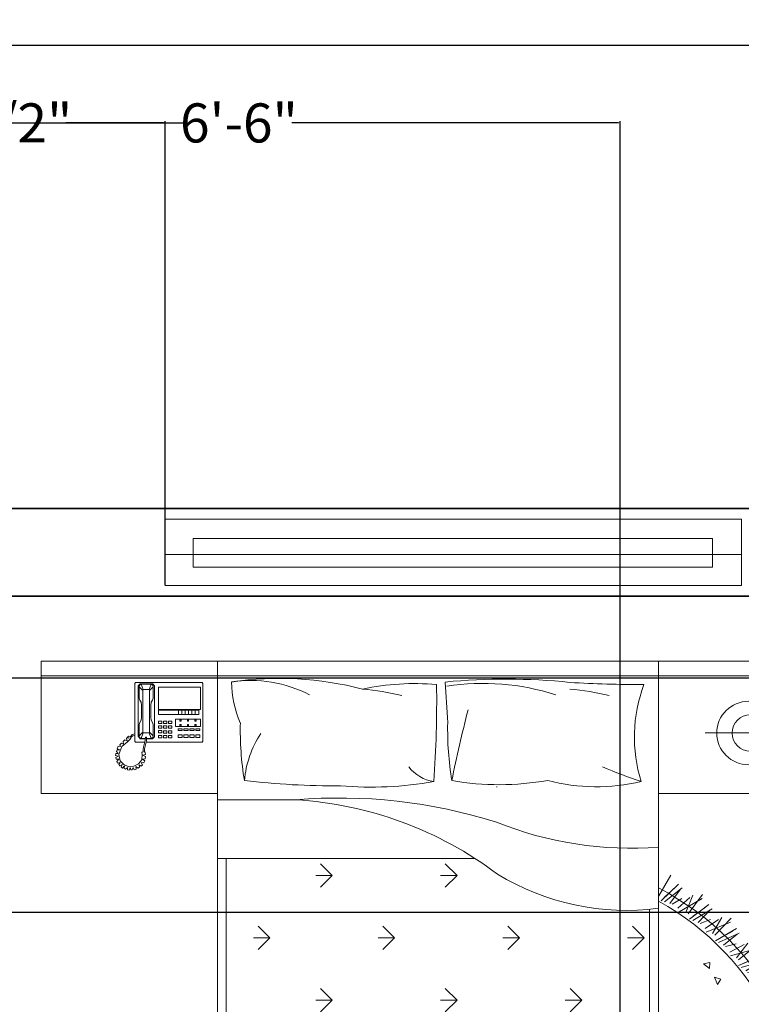
# Model space of a CAD drawing. Units: inches. Extents: x 311 to 754, y 60 to 497.
# Tile 4 of 11: x 388 to 462, y 396 to 497. Entities that reach past the tile are written whole.
import ezdxf

# ---------------------------------------------------------------- set-up
doc = ezdxf.new("R2010")
doc.units = ezdxf.units.IN
doc.header["$MEASUREMENT"] = 0
for name, color, linetype, lineweight in [('A-ANNO-DIMS', 2, 'Continuous', 18), ('A-WALL', 7, 'Continuous', 35), ('beds', 70, 'Continuous', 13), ('windows', 120, 'Continuous', 18)]:
    doc.layers.add(name, color=color, linetype=linetype, lineweight=lineweight)
doc.styles.get("Standard").update_dxf_attribs({"font": 'arial.ttf'})
doc.dimstyles.get("Standard").update_dxf_attribs({"dimtxt": 4, "dimasz": 0.18, "dimexe": 0.18, "dimexo": 0.0625, "dimgap": 0.09, "dimtad": 0, "dimtih": 1, "dimtoh": 1, "dimdec": 0, "dimrnd": 6, "dimzin": 0, "dimdsep": 46, "dimlunit": 3, "dimtxsty": 'Standard', "dimcen": 0.09, "dimadec": 0, "dimazin": 0, "dimtfac": 1, "dimtdec": 0, "dimtofl": 0, "dimtmove": 0, "dimatfit": 3, "dimfxl": 1, "dimtolj": 1, "dimtzin": 0, "dimarcsym": 0})

# ---------------------------------------------------------------- blocks, each defined once
blk = doc.blocks.new('A$C57792D97')
for p, q in [((0.6, 2.6235), (0, 2.6235)), ((0, 2.6235), (0, 2.1735)), ((2.1, 2.6235), (0.6, 2.6235)), ((0.6, 2.6235), (0.6, 0.6235)), ((0.6, 0.6235), (0.6, 2.6235)), ((0.6, 2.1735), (0.6, 2.6235)), ((2.1, 0.6235), (2.1, 2.6235)), ((2.7, 2.6235), (2.1, 2.6235)), ((2.1, 2.6235), (2.1, 2.1735)), ((2.7, 2.1735), (2.7, 2.6235)), ((0.6, 2.5735), (0, 2.5735)), ((2.1, 2.5735), (0.6, 2.5735)), ((2.7, 2.5735), (2.1, 2.5735)), ((2.4103, 2.2312), (2.4103, 2.5317)), ((2.2593, 2.3802), (2.5698, 2.3802)), ((1.5491, 2.1955), (1.5516, 2.1955)), ((0, 2.1735), (0.6, 2.1735)), ((0.6, 2.1518), (0.8661, 2.1518)), ((2.1, 2.1735), (2.7, 2.1735)), ((0.6, 1.9518), (1.4767, 1.9518)), ((0.63, 0.6535), (0.63, 1.9518)), ((0.9906, 1.8942), (0.9508, 1.934)), ((1.4149, 1.8942), (1.3751, 1.934)), ((0.9906, 1.8942), (0.9344, 1.8942)), ((0.9906, 1.8942), (0.9508, 1.8544)), ((1.4149, 1.8942), (1.3586, 1.8942)), ((1.4149, 1.8942), (1.3751, 1.8544)), ((2.142, 1.8959), (2.1018, 1.8254)), ((2.1679, 1.8652), (2.1088, 1.8077)), ((2.1584, 1.8544), (2.1201, 1.8188)), ((2.1812, 1.8524), (2.1207, 1.8046)), ((2.1749, 1.8475), (2.1394, 1.7993)), ((2.1799, 1.8155), (2.1465, 1.7971)), ((2.2066, 1.8191), (2.1664, 1.7827)), ((2.249, 1.8154), (2.1711, 1.7709)), ((2.2173, 1.8274), (2.1931, 1.7688)), ((2.2496, 1.8292), (2.2008, 1.7642)), ((2.07, 1.7793), (2.07, 0.6535)), ((2.2713, 1.7954), (2.2055, 1.7458)), ((2.283, 1.7811), (2.2169, 1.7413)), ((2.2607, 1.7859), (2.2181, 1.7554)), ((2.2761, 1.777), (2.2348, 1.7337)), ((2.277, 1.7446), (2.2416, 1.7306)), ((2.304, 1.7449), (2.2596, 1.7138)), ((2.3157, 1.7518), (2.2843, 1.6966)), ((2.3479, 1.7495), (2.2914, 1.6911)), ((0.7785, 1.6821), (0.7387, 1.7219)), ((1.2027, 1.6821), (1.163, 1.7219)), ((1.627, 1.6821), (1.5872, 1.7219)), ((2.0513, 1.6821), (2.0115, 1.7219)), ((2.3456, 1.7359), (2.2627, 1.7015)), ((2.3653, 1.7133), (2.2937, 1.6723)), ((0.7785, 1.6821), (0.7222, 1.6821)), ((0.7785, 1.6821), (0.7387, 1.6423)), ((1.2027, 1.6821), (1.1465, 1.6821)), ((1.2027, 1.6821), (1.163, 1.6423)), ((1.627, 1.6821), (1.5708, 1.6821)), ((1.627, 1.6821), (1.5872, 1.6423)), ((2.0513, 1.6821), (1.995, 1.6821)), ((2.0513, 1.6821), (2.0115, 1.6423)), ((2.3751, 1.6976), (2.3045, 1.6664)), ((2.3535, 1.7051), (2.3075, 1.6802)), ((2.3677, 1.6944), (2.3213, 1.6565)), ((2.3645, 1.6621), (2.3277, 1.6526)), ((2.3913, 1.659), (2.3434, 1.6337)), ((2.4314, 1.6449), (2.3449, 1.6211)), ((2.4038, 1.6644), (2.3657, 1.6136)), ((2.4355, 1.6581), (2.372, 1.6073)), ((2.4482, 1.62), (2.372, 1.5882)), ((2.4354, 1.6134), (2.3867, 1.5944)), ((2.2754, 1.598), (2.2534, 1.5939)), ((2.2736, 1.5771), (2.2535, 1.594)), ((2.2736, 1.5771), (2.2754, 1.598)), ((2.4559, 1.6032), (2.382, 1.581)), ((2.4482, 1.6009), (2.3974, 1.5692)), ((2.3123, 1.541), (2.2911, 1.5481)), ((2.3006, 1.5236), (2.2912, 1.5481)), ((2.441, 1.5693), (2.4032, 1.5645)), ((2.4672, 1.5629), (2.4164, 1.5438)), ((2.5052, 1.5438), (2.4164, 1.5311)), ((2.4802, 1.5667), (2.4361, 1.5211)), ((2.5109, 1.5564), (2.4416, 1.514)), ((0.9906, 1.47), (0.9508, 1.5097)), ((1.4149, 1.47), (1.3751, 1.5097)), ((1.8391, 1.47), (1.7994, 1.5097)), ((2.3006, 1.5236), (2.3123, 1.541)), ((2.5187, 1.517), (2.4392, 1.4951)), ((2.5052, 1.5121), (2.4545, 1.4994)), ((2.5243, 1.4994), (2.4482, 1.4867)), ((2.5163, 1.4981), (2.462, 1.473)), ((0.9906, 1.47), (0.9344, 1.47)), ((0.9906, 1.47), (0.9508, 1.4302)), ((1.4149, 1.47), (1.3586, 1.47)), ((1.4149, 1.47), (1.3751, 1.4302)), ((1.8391, 1.47), (1.7829, 1.47)), ((1.8391, 1.47), (1.7994, 1.4302)), ((2.5052, 1.4677), (2.4672, 1.4677)), ((2.5304, 1.458), (2.4777, 1.4454)), ((2.5438, 1.4601), (2.4943, 1.4204)), ((2.573, 1.4461), (2.4989, 1.4127)), ((2.5658, 1.4343), (2.4761, 1.4328)), ((2.5758, 1.406), (2.4942, 1.3942)), ((2.5791, 1.3878), (2.502, 1.3848)), ((2.5618, 1.4028), (2.5099, 1.3966)), ((2.571, 1.3876), (2.514, 1.3695)), ((2.2534, 1.3469), (2.2315, 1.3429)), ((2.2516, 1.326), (2.2315, 1.3429)), ((2.2516, 1.326), (2.2535, 1.347)), ((2.5562, 1.3587), (2.5185, 1.3635)), ((2.58, 1.346), (2.5261, 1.3402)), ((2.5936, 1.3464), (2.5395, 1.3132)), ((2.1596, 1.3147), (2.1502, 1.3392)), ((2.1714, 1.3321), (2.1502, 1.3392)), ((2.1596, 1.3147), (2.1714, 1.3321)), ((2.3632, 1.3229), (2.33, 1.319)), ((2.3584, 1.2918), (2.33, 1.319)), ((2.3584, 1.2918), (2.3632, 1.3229)), ((2.6121, 1.3181), (2.523, 1.3279)), ((2.6207, 1.3289), (2.5431, 1.305)), ((0.7785, 1.2578), (0.7387, 1.2976)), ((1.2027, 1.2578), (1.163, 1.2976)), ((1.627, 1.2578), (1.5872, 1.2976)), ((2.0513, 1.2578), (2.0115, 1.2976)), ((2.6185, 1.2888), (2.5361, 1.2873)), ((2.6195, 1.2703), (2.5426, 1.277)), ((2.6042, 1.2873), (2.5519, 1.2877)), ((0.7785, 1.2578), (0.7222, 1.2578)), ((0.7785, 1.2578), (0.7387, 1.218)), ((1.2027, 1.2578), (1.1465, 1.2578)), ((1.2027, 1.2578), (1.163, 1.218)), ((1.627, 1.2578), (1.5708, 1.2578)), ((1.627, 1.2578), (1.5872, 1.218)), ((2.0513, 1.2578), (1.995, 1.2578)), ((2.0513, 1.2578), (2.0115, 1.218)), ((2.4134, 1.2295), (2.404, 1.254)), ((2.4252, 1.2469), (2.404, 1.254)), ((2.4134, 1.2295), (2.4252, 1.2469)), ((2.6115, 1.2711), (2.5526, 1.2603)), ((2.5932, 1.2443), (2.5563, 1.2538)), ((2.6435, 1.197), (2.5563, 1.2178)), ((2.6152, 1.2287), (2.561, 1.2296)), ((2.6287, 1.2274), (2.5709, 1.2013)), ((2.6462, 1.1671), (2.5642, 1.176)), ((2.6534, 1.2066), (2.5734, 1.1926)), ((2.6319, 1.1675), (2.58, 1.1743)), ((2.4947, 1.1445), (2.4728, 1.1404)), ((2.4929, 1.1236), (2.4728, 1.1404)), ((2.4929, 1.1236), (2.4948, 1.1445)), ((2.6449, 1.1486), (2.5694, 1.1649)), ((2.637, 1.1504), (2.5773, 1.147)), ((2.6155, 1.1261), (2.5801, 1.1402)), ((2.6353, 1.1079), (2.5817, 1.1156)), ((0.9906, 1.0457), (0.9508, 1.0855)), ((1.4149, 1.0457), (1.3751, 1.0855)), ((1.8391, 1.0457), (1.7994, 1.0855)), ((2.2315, 1.0959), (2.2095, 1.0919)), ((2.2297, 1.075), (2.2096, 1.0919)), ((2.2297, 1.075), (2.2315, 1.0959)), ((2.6595, 1.0729), (2.5756, 1.1045)), ((2.6486, 1.1049), (2.588, 1.0862)), ((2.6705, 1.0812), (2.5894, 1.0774)), ((0.9906, 1.0457), (0.9344, 1.0457)), ((0.9906, 1.0457), (0.9508, 1.0059)), ((1.4149, 1.0457), (1.3586, 1.0457)), ((1.4149, 1.0457), (1.3751, 1.0059)), ((1.8391, 1.0457), (1.7829, 1.0457)), ((1.8391, 1.0457), (1.7994, 1.0059)), ((2.2725, 1.0206), (2.2631, 1.0451)), ((2.2842, 1.038), (2.2631, 1.0451)), ((2.6584, 1.0429), (2.5782, 1.062)), ((2.6548, 1.0248), (2.582, 1.0503)), ((2.6442, 1.045), (2.5937, 1.0584)), ((2.2725, 1.0206), (2.2843, 1.038)), ((2.6472, 1.0275), (2.5875, 1.0316)), ((2.6228, 1.0061), (2.5895, 1.0244)), ((2.6598, 0.9477), (2.5805, 0.9897)), ((2.6402, 0.9855), (2.588, 0.9999)), ((2.653, 0.9809), (2.5905, 0.97)), ((2.3053, 0.9493), (2.272, 0.9455)), ((2.3005, 0.9182), (2.2721, 0.9455)), ((2.3005, 0.9182), (2.3053, 0.9494)), ((2.5263, 0.9355), (2.5169, 0.96)), ((2.538, 0.9528), (2.5169, 0.9599)), ((2.5263, 0.9355), (2.5381, 0.9529)), ((2.655, 0.9181), (2.5778, 0.9471)), ((2.6718, 0.9546), (2.5908, 0.961)), ((2.6412, 0.9221), (2.5927, 0.9416)), ((2.6491, 0.9006), (2.5801, 0.9351)), ((2.6419, 0.9043), (2.5832, 0.9159)), ((2.6151, 0.8861), (2.5843, 0.9085)), ((0.7785, 0.8336), (0.7387, 0.8733)), ((1.2027, 0.8336), (1.163, 0.8733)), ((1.627, 0.8336), (1.5872, 0.8733)), ((2.0513, 0.8336), (2.0115, 0.8733)), ((2.4728, 0.8934), (2.4508, 0.8894)), ((2.471, 0.8725), (2.4509, 0.8894)), ((2.471, 0.8725), (2.4728, 0.8934)), ((2.6444, 0.8236), (2.571, 0.8751)), ((2.6297, 0.8635), (2.5797, 0.8843)), ((2.2095, 0.8449), (2.1876, 0.8408)), ((2.2077, 0.824), (2.1876, 0.8408)), ((2.2077, 0.824), (2.2095, 0.8449)), ((2.6572, 0.8289), (2.5776, 0.8454)), ((2.6418, 0.8573), (2.5785, 0.8543)), ((0.7785, 0.8336), (0.7222, 0.8336)), ((0.7785, 0.8336), (0.7387, 0.7938)), ((1.2027, 0.8336), (1.1465, 0.8336)), ((1.2027, 0.8336), (1.163, 0.7938)), ((1.627, 0.8336), (1.5708, 0.8336)), ((1.627, 0.8336), (1.5872, 0.7938)), ((2.0513, 0.8336), (1.995, 0.8336)), ((2.0513, 0.8336), (2.0115, 0.7938)), ((2.1316, 0.8117), (2.1222, 0.8362)), ((2.1433, 0.8291), (2.1222, 0.8362)), ((2.1316, 0.8117), (2.1434, 0.8291)), ((2.6359, 0.7948), (2.5629, 0.8332)), ((2.6279, 0.7781), (2.5637, 0.821)), ((2.6227, 0.8004), (2.577, 0.8259)), ((1.9462, 0.7963), (1.9243, 0.7923)), ((2.6212, 0.7827), (2.5644, 0.8015)), ((2.5923, 0.768), (2.5646, 0.7941)), ((1.683, 0.7477), (1.661, 0.7437)), ((2.3854, 0.7265), (2.376, 0.751)), ((2.3971, 0.7439), (2.376, 0.751)), ((2.3854, 0.7265), (2.3972, 0.7439)), ((2.6136, 0.7023), (2.5472, 0.7626)), ((2.6153, 0.7361), (2.552, 0.7411)), ((2.604, 0.7437), (2.557, 0.7707)), ((2.5915, 0.6593), (2.5332, 0.7099)), ((2.6016, 0.6748), (2.534, 0.7221)), ((2.5892, 0.6821), (2.547, 0.7131)), ((2.6269, 0.706), (2.5501, 0.7323)), ((1.4197, 0.6992), (1.3978, 0.6951)), ((2.5549, 0.6537), (2.5307, 0.6831)), ((2.5855, 0.6646), (2.5315, 0.6905)), ((0.9906, 0.6214), (0.9508, 0.6612)), ((1.1564, 0.6506), (1.1345, 0.6466)), ((1.4149, 0.6214), (1.3751, 0.6612)), ((1.8391, 0.6214), (1.7994, 0.6612)), ((2.4508, 0.6424), (2.4289, 0.6383)), ((2.449, 0.6215), (2.4289, 0.6384)), ((2.449, 0.6215), (2.4508, 0.6424)), ((2.5678, 0.5858), (2.5095, 0.654)), ((2.5635, 0.6282), (2.5203, 0.6608)), ((2.02, 0.6035), (0.6716, 0.6035)), ((0.9906, 0.6214), (0.9344, 0.6214)), ((0.9906, 0.6214), (0.9727, 0.6035)), ((1.4149, 0.6214), (1.3586, 0.6214)), ((1.4149, 0.6214), (1.397, 0.6035)), ((1.8391, 0.6214), (1.7829, 0.6214)), ((1.8391, 0.6214), (1.8212, 0.6035)), ((2.5405, 0.546), (2.489, 0.6034)), ((2.5524, 0.5601), (2.4913, 0.6155)), ((2.541, 0.5688), (2.5031, 0.6049)), ((2.5815, 0.5878), (2.5085, 0.6236)), ((2.5737, 0.6192), (2.5116, 0.632)), ((0.6417, 0.5735), (2.05, 0.5735)), ((0.8932, 0.6021), (0.8712, 0.598)), ((1.3422, 0.5642), (1.3386, 0.5735)), ((1.3422, 0.5642), (1.3485, 0.5735)), ((2.1875, 0.5938), (2.1656, 0.5898)), ((2.1857, 0.5729), (2.1656, 0.5898)), ((2.1857, 0.5729), (2.1876, 0.5938)), ((2.2473, 0.5758), (2.2141, 0.5719)), ((2.2425, 0.5447), (2.2141, 0.572)), ((2.2425, 0.5447), (2.2474, 0.5758)), ((2.5035, 0.545), (2.4831, 0.5772)), ((2.5352, 0.552), (2.4849, 0.5844)), ((0.8142, 0.5177), (0.8685, 0.5428)), ((1.9243, 0.5453), (1.9023, 0.5412)), ((1.9225, 0.5244), (1.9024, 0.5412)), ((1.9225, 0.5244), (1.9243, 0.5453)), ((2.2445, 0.5176), (2.2351, 0.5421)), ((2.5078, 0.476), (2.4585, 0.551)), ((2.5088, 0.5186), (2.47, 0.5564)), ((0.8062, 0.5164), (0.8823, 0.5291)), ((0.8118, 0.4988), (0.8913, 0.5207)), ((0.8253, 0.5037), (0.876, 0.5164)), ((1.6077, 0.4964), (1.5865, 0.5035)), ((1.596, 0.479), (1.5866, 0.5035)), ((1.8485, 0.5294), (1.8152, 0.5255)), ((1.8437, 0.4983), (1.8153, 0.5256)), ((1.8437, 0.4983), (1.8485, 0.5294)), ((2.2445, 0.5176), (2.2562, 0.535)), ((2.4757, 0.4399), (2.4318, 0.5034)), ((2.4893, 0.4525), (2.4356, 0.515)), ((2.4791, 0.4625), (2.446, 0.503)), ((2.5216, 0.4763), (2.4537, 0.5209)), ((2.5178, 0.5084), (2.4578, 0.5289)), ((0.8196, 0.4594), (0.8889, 0.5018)), ((0.8253, 0.472), (0.9141, 0.4847)), ((0.8503, 0.4491), (0.8944, 0.4947)), ((0.8633, 0.4529), (0.9141, 0.472)), ((1.4496, 0.483), (1.4163, 0.4791)), ((1.4448, 0.4519), (1.4164, 0.4792)), ((1.4448, 0.4519), (1.4496, 0.483)), ((1.596, 0.479), (1.6077, 0.4964)), ((1.661, 0.4967), (1.6391, 0.4927)), ((1.6592, 0.4758), (1.6391, 0.4927)), ((1.6592, 0.4758), (1.661, 0.4967)), ((2.4389, 0.4436), (2.4227, 0.478)), ((2.4712, 0.4466), (2.4253, 0.485)), ((0.8823, 0.4149), (0.9331, 0.4466)), ((0.8895, 0.4465), (0.9273, 0.4513)), ((0.9592, 0.4578), (0.938, 0.4649)), ((0.9403, 0.459), (0.9381, 0.4649)), ((0.9508, 0.4454), (0.9592, 0.4578)), ((1.0507, 0.4366), (1.0175, 0.4327)), ((1.0459, 0.4055), (1.0507, 0.4366)), ((1.3977, 0.4481), (1.3758, 0.4441)), ((1.3959, 0.4272), (1.3758, 0.4441)), ((1.3959, 0.4272), (1.3978, 0.4482)), ((2.4345, 0.3746), (2.395, 0.4552)), ((2.4409, 0.4167), (2.4071, 0.4591)), ((0.8746, 0.4126), (0.9485, 0.4347)), ((0.8823, 0.3958), (0.9585, 0.4275)), ((0.895, 0.3577), (0.9585, 0.4085)), ((0.8951, 0.4024), (0.9438, 0.4214)), ((1.0459, 0.4055), (1.0175, 0.4328)), ((1.8615, 0.4113), (1.8403, 0.4184)), ((1.8498, 0.3939), (1.8404, 0.4184)), ((1.8498, 0.3939), (1.8615, 0.4113)), ((2.3981, 0.3428), (2.3625, 0.4113)), ((2.4132, 0.3535), (2.3678, 0.4224)), ((2.4043, 0.3648), (2.3766, 0.4092)), ((2.4482, 0.3731), (2.3865, 0.4259)), ((2.4485, 0.4055), (2.3915, 0.4334)), ((0.8991, 0.3709), (0.9856, 0.3946)), ((0.9267, 0.3514), (0.9648, 0.4022)), ((0.9392, 0.3568), (0.9872, 0.3821)), ((1.1345, 0.3996), (1.1125, 0.3955)), ((1.1327, 0.3787), (1.1126, 0.3955)), ((1.1327, 0.3787), (1.1345, 0.3996)), ((1.213, 0.3727), (1.1918, 0.3798)), ((1.2013, 0.3553), (1.1919, 0.3798)), ((1.2013, 0.3553), (1.213, 0.3727)), ((2.3607, 0.3242), (2.3324, 0.3704)), ((2.3621, 0.3511), (2.3503, 0.3873)), ((2.3945, 0.35), (2.3538, 0.3939)), ((0.9555, 0.3182), (1.026, 0.3494)), ((0.9628, 0.3214), (1.0092, 0.3592)), ((0.9652, 0.3025), (1.0368, 0.3435)), ((0.966, 0.3537), (1.0029, 0.3631)), ((0.977, 0.3107), (1.023, 0.3356)), ((2.1656, 0.3428), (2.1436, 0.3387)), ((2.1638, 0.3219), (2.1437, 0.3388)), ((2.1638, 0.3219), (2.1656, 0.3428)), ((2.3253, 0.265), (2.2888, 0.3389)), ((2.3625, 0.28), (2.3078, 0.3401)), ((2.3668, 0.3121), (2.3138, 0.3469)), ((2.3491, 0.2832), (2.32, 0.3681)), ((0.9826, 0.2663), (1.0392, 0.3246)), ((0.9849, 0.2799), (1.0678, 0.3143)), ((1.0148, 0.264), (1.0462, 0.3191)), ((1.0265, 0.2709), (1.0709, 0.302)), ((2.1153, 0.3261), (2.0941, 0.3332)), ((2.1036, 0.3087), (2.0942, 0.3332)), ((2.1036, 0.3087), (2.1153, 0.3261)), ((2.2743, 0.2689), (2.2671, 0.3063)), ((2.3063, 0.2638), (2.2714, 0.3124)), ((2.309, 0.2562), (2.2823, 0.3286)), ((2.3179, 0.2773), (2.2959, 0.3247)), ((1.0475, 0.2347), (1.1136, 0.2745)), ((1.0535, 0.2712), (1.0889, 0.2852)), ((1.0544, 0.2388), (1.0957, 0.2821)), ((1.0592, 0.2203), (1.125, 0.27)), ((1.4668, 0.2875), (1.4456, 0.2946)), ((1.4551, 0.2701), (1.4457, 0.2946)), ((1.4551, 0.2701), (1.4668, 0.2875)), ((1.9023, 0.2942), (1.8804, 0.2902)), ((1.9005, 0.2733), (1.8804, 0.2902)), ((1.9005, 0.2733), (1.9023, 0.2942)), ((2.2741, 0.2296), (2.2258, 0.2708)), ((2.2529, 0.2032), (2.2346, 0.291)), ((2.2695, 0.2424), (2.2473, 0.2918)), ((1.0699, 0.2299), (1.1124, 0.2604)), ((1.0809, 0.1866), (1.1297, 0.2516)), ((1.0815, 0.2004), (1.1594, 0.2449)), ((1.1132, 0.1884), (1.1374, 0.247)), ((1.639, 0.2457), (1.6171, 0.2416)), ((1.6372, 0.2248), (1.6171, 0.2416)), ((1.6372, 0.2248), (1.6391, 0.2457)), ((2.1768, 0.1984), (2.1745, 0.2364)), ((2.208, 0.1893), (2.1795, 0.2419)), ((2.2097, 0.1814), (2.1923, 0.2566)), ((2.227, 0.1881), (2.2001, 0.2661)), ((2.2212, 0.2012), (2.2053, 0.2511)), ((2.2658, 0.1984), (2.2191, 0.2649)), ((1.1239, 0.1967), (1.1641, 0.2331)), ((1.1493, 0.1634), (1.2098, 0.2112)), ((1.1507, 0.2003), (1.184, 0.2187)), ((1.1556, 0.1683), (1.1911, 0.2165)), ((1.1626, 0.1506), (1.2217, 0.2081)), ((1.7206, 0.2023), (1.6994, 0.2094)), ((1.7089, 0.1849), (1.6995, 0.2095)), ((1.7089, 0.1849), (1.7206, 0.2024)), ((2.1198, 0.1242), (2.1029, 0.2049)), ((2.1596, 0.1295), (2.1216, 0.2013)), ((2.1718, 0.1594), (2.129, 0.2063)), ((2.1474, 0.1359), (2.1403, 0.2253)), ((2.1688, 0.1727), (2.1529, 0.2245)), ((1.1721, 0.1614), (1.2104, 0.197)), ((1.1873, 0.1336), (1.259, 0.1875)), ((1.1885, 0.1199), (1.2287, 0.1904)), ((1.2203, 0.1256), (1.237, 0.1868)), ((1.2299, 0.1352), (1.2652, 0.1764)), ((1.3758, 0.1971), (1.3538, 0.193)), ((1.374, 0.1762), (1.3539, 0.1931)), ((1.374, 0.1762), (1.3758, 0.1971)), ((2.0343, 0.0824), (2.0385, 0.172)), ((2.0601, 0.1162), (2.0509, 0.1696)), ((2.0714, 0.1407), (2.0737, 0.1787)), ((2.1011, 0.1277), (2.0794, 0.1835)), ((2.1018, 0.1197), (2.0939, 0.1965)), ((2.1157, 0.1379), (2.1062, 0.1893)), ((1.2559, 0.1422), (1.2867, 0.1646)), ((1.2592, 0.1054), (1.3133, 0.1604)), ((1.2649, 0.111), (1.2941, 0.1633)), ((1.2741, 0.0944), (1.3255, 0.1588)), ((1.282, 0.1063), (1.3156, 0.1464)), ((1.3007, 0.0806), (1.3651, 0.1431)), ((1.3035, 0.0671), (1.3346, 0.1421)), ((1.3344, 0.0768), (1.3433, 0.1396)), ((1.7905, 0.1559), (1.7573, 0.152)), ((1.7857, 0.1248), (1.7573, 0.152)), ((1.7857, 0.1248), (1.7906, 0.1559)), ((1.9873, 0.08), (1.9728, 0.1381)), ((1.9871, 0.072), (1.9889, 0.1491)), ((2.0054, 0.0742), (1.9988, 0.1564)), ((2.0031, 0.0883), (2.0001, 0.1405)), ((2.0456, 0.0745), (2.0169, 0.1505)), ((2.0614, 0.1027), (2.0249, 0.1545)), ((1.3427, 0.0876), (1.3725, 0.1328)), ((1.3677, 0.0977), (1.3954, 0.1238)), ((1.3755, 0.0616), (1.4223, 0.1229)), ((1.3804, 0.0679), (1.4028, 0.1234)), ((1.3916, 0.0525), (1.4346, 0.1229)), ((1.3981, 0.0653), (1.4264, 0.1093)), ((1.4198, 0.0422), (1.4758, 0.1123)), ((1.4243, 0.0292), (1.4458, 0.1075)), ((1.4537, 0.0427), (1.4546, 0.1061)), ((1.4606, 0.0544), (1.4845, 0.103)), ((1.5135, 0.0258), (1.5473, 0.101)), ((1.7925, 0.0197), (1.8188, 0.1054)), ((1.8429, 0.0669), (1.8547, 0.1031)), ((1.8685, 0.047), (1.8614, 0.1064)), ((1.8672, 0.039), (1.8787, 0.1154)), ((1.8852, 0.0532), (1.8888, 0.1054)), ((1.8857, 0.0389), (1.8894, 0.1213)), ((1.9256, 0.0342), (1.9067, 0.1132)), ((1.9448, 0.0601), (1.9151, 0.1162)), ((1.9154, 0.0434), (1.9307, 0.1318)), ((1.9452, 0.0737), (1.9428, 0.1279)), ((1.9595, 0.0966), (1.9666, 0.134)), ((1.4841, 0.0676), (1.5083, 0.0969)), ((1.4964, 0.0327), (1.5351, 0.0995)), ((1.5005, 0.0397), (1.5158, 0.0975)), ((1.5183, 0.0393), (1.5409, 0.0865)), ((1.5428, 0.0191), (1.5896, 0.0956)), ((1.5489, 0.0067), (1.5603, 0.0871)), ((1.5763, 0.0238), (1.5693, 0.0868)), ((1.5817, 0.0362), (1.5994, 0.0875)), ((1.6034, 0.0523), (1.6237, 0.0845)), ((1.6199, 0.0192), (1.65, 0.0903)), ((1.6232, 0.0266), (1.631, 0.086)), ((1.6378, 0.0145), (1.6619, 0.0934)), ((1.6409, 0.0285), (1.6573, 0.0782)), ((1.6677, 0.0115), (1.7045, 0.0933)), ((1.6753, 0), (1.6766, 0.0812)), ((1.7004, 0.0204), (1.6855, 0.0821)), ((1.7041, 0.0334), (1.7152, 0.0865)), ((1.7236, 0.0521), (1.7398, 0.0865)), ((1.7442, 0.0214), (1.7651, 0.0956)), ((1.7465, 0.0291), (1.7469, 0.0889)), ((1.7625, 0.0189), (1.7765, 0.1002)), ((1.7638, 0.0332), (1.7739, 0.0845)), ((1.8015, 0.0092), (1.7926, 0.09)), ((1.8238, 0.0326), (1.8014, 0.0919)), ((1.8259, 0.046), (1.8303, 0.1))]:
    blk.add_line(p, q)
at = {"linetype": 'ByBlock'}
for p, q in [((0.3217, 2.5511), (0.3189, 2.5483)), ((0.3189, 2.5483), (0.3189, 2.3511)), ((0.5475, 2.5511), (0.3217, 2.5511)), ((0.5475, 2.5511), (0.5503, 2.5483)), ((0.5503, 2.5483), (0.5503, 2.3511)), ((0.3375, 2.5469), (0.3303, 2.5397)), ((0.3303, 2.5397), (0.3303, 2.3683)), ((0.3346, 2.5426), (0.3332, 2.5369)), ((0.3332, 2.5369), (0.3332, 2.4983)), ((0.3332, 2.5369), (0.346, 2.524)), ((0.3403, 2.5454), (0.3346, 2.5426)), ((0.3803, 2.5469), (0.3375, 2.5469)), ((0.3746, 2.5454), (0.3403, 2.5454)), ((0.3475, 2.5269), (0.3403, 2.5454)), ((0.346, 2.524), (0.3475, 2.5269)), ((0.346, 2.4597), (0.346, 2.524)), ((0.3475, 2.5269), (0.3675, 2.5269)), ((0.3675, 2.5269), (0.3746, 2.5454)), ((0.3689, 2.524), (0.3675, 2.5269)), ((0.3818, 2.5369), (0.3689, 2.524)), ((0.3689, 2.4597), (0.3689, 2.524)), ((0.3746, 2.5454), (0.3803, 2.5426)), ((0.386, 2.5397), (0.3803, 2.5469)), ((0.3803, 2.5426), (0.3818, 2.5369)), ((0.3818, 2.5369), (0.3818, 2.4983)), ((0.386, 2.3668), (0.386, 2.5397)), ((0.3989, 2.4597), (0.3989, 2.5354)), ((0.3989, 2.5354), (0.5418, 2.5354)), ((0.5418, 2.5354), (0.5418, 2.4597)), ((0.3332, 2.4983), (0.336, 2.4911)), ((0.336, 2.4911), (0.3403, 2.484)), ((0.3403, 2.484), (0.3417, 2.474)), ((0.3746, 2.484), (0.3732, 2.474)), ((0.3789, 2.4911), (0.3746, 2.484)), ((0.3818, 2.4983), (0.3789, 2.4911)), ((0.3417, 2.474), (0.3417, 2.4597)), ((0.3417, 2.4326), (0.3417, 2.4597)), ((0.346, 2.4597), (0.346, 2.3826)), ((0.3689, 2.4597), (0.3689, 2.3826)), ((0.3732, 2.474), (0.3732, 2.4597)), ((0.3732, 2.4326), (0.3732, 2.4597)), ((0.5418, 2.4597), (0.3989, 2.4597)), ((0.3989, 2.4426), (0.3989, 2.4568)), ((0.3989, 2.4568), (0.5361, 2.4568)), ((0.4675, 2.4568), (0.4675, 2.4426)), ((0.4789, 2.4568), (0.4789, 2.4426)), ((0.4903, 2.4568), (0.4903, 2.4426)), ((0.5018, 2.4568), (0.5018, 2.4426)), ((0.5132, 2.4568), (0.5132, 2.4426)), ((0.5246, 2.4568), (0.5246, 2.4426)), ((0.5361, 2.4568), (0.5361, 2.4426)), ((0.3332, 2.4083), (0.336, 2.4154)), ((0.336, 2.4154), (0.3403, 2.4226)), ((0.3403, 2.4226), (0.3417, 2.4326)), ((0.3746, 2.4226), (0.3732, 2.4326)), ((0.3789, 2.4154), (0.3746, 2.4226)), ((0.3818, 2.4083), (0.3789, 2.4154)), ((0.5361, 2.4426), (0.3989, 2.4426)), ((0.3989, 2.4197), (0.3989, 2.4111)), ((0.4103, 2.4197), (0.3989, 2.4197)), ((0.4103, 2.4111), (0.4103, 2.4197)), ((0.4275, 2.4197), (0.416, 2.4197)), ((0.416, 2.4197), (0.416, 2.4111)), ((0.4275, 2.4111), (0.4275, 2.4197)), ((0.4332, 2.4197), (0.4332, 2.4111)), ((0.4446, 2.4197), (0.4332, 2.4197)), ((0.4446, 2.4111), (0.4446, 2.4197)), ((0.4575, 2.4011), (0.4575, 2.4268)), ((0.4575, 2.4268), (0.5418, 2.4268)), ((0.4718, 2.424), (0.4761, 2.424)), ((0.4718, 2.4197), (0.4718, 2.424)), ((0.4761, 2.4197), (0.4718, 2.4197)), ((0.4761, 2.424), (0.4761, 2.4197)), ((0.4975, 2.424), (0.5018, 2.424)), ((0.4975, 2.4197), (0.4975, 2.424)), ((0.5018, 2.4197), (0.4975, 2.4197)), ((0.5018, 2.424), (0.5018, 2.4197)), ((0.5232, 2.4197), (0.5232, 2.424)), ((0.5232, 2.424), (0.5275, 2.424)), ((0.5275, 2.4197), (0.5232, 2.4197)), ((0.5275, 2.424), (0.5275, 2.4197)), ((0.5418, 2.4268), (0.5418, 2.4011)), ((0.3332, 2.3697), (0.3332, 2.4083)), ((0.3332, 2.3697), (0.346, 2.3826)), ((0.3475, 2.3797), (0.3403, 2.3611)), ((0.346, 2.3826), (0.3475, 2.3797)), ((0.3475, 2.3797), (0.3675, 2.3797)), ((0.3689, 2.3826), (0.3675, 2.3797)), ((0.3675, 2.3797), (0.3746, 2.3611)), ((0.3818, 2.3697), (0.3689, 2.3826)), ((0.3818, 2.3697), (0.3818, 2.4083)), ((0.3989, 2.4111), (0.4103, 2.4111)), ((0.3989, 2.404), (0.3989, 2.3954)), ((0.4103, 2.404), (0.3989, 2.404)), ((0.3989, 2.3954), (0.4103, 2.3954)), ((0.4103, 2.3883), (0.3989, 2.3883)), ((0.3989, 2.3883), (0.3989, 2.3797)), ((0.3989, 2.3797), (0.4103, 2.3797)), ((0.4103, 2.3954), (0.4103, 2.404)), ((0.4103, 2.3797), (0.4103, 2.3883)), ((0.416, 2.4111), (0.4275, 2.4111)), ((0.416, 2.404), (0.416, 2.3954)), ((0.4275, 2.404), (0.416, 2.404)), ((0.416, 2.3954), (0.4275, 2.3954)), ((0.4275, 2.3868), (0.416, 2.3868)), ((0.416, 2.3868), (0.416, 2.3783)), ((0.4275, 2.3954), (0.4275, 2.404)), ((0.4275, 2.3783), (0.4275, 2.3868)), ((0.4332, 2.4111), (0.4446, 2.4111)), ((0.4332, 2.404), (0.4332, 2.3954)), ((0.4446, 2.404), (0.4332, 2.404)), ((0.4332, 2.3954), (0.4446, 2.3954)), ((0.4446, 2.3868), (0.4332, 2.3868)), ((0.4332, 2.3868), (0.4332, 2.3783)), ((0.4446, 2.3954), (0.4446, 2.404)), ((0.4446, 2.3783), (0.4446, 2.3868)), ((0.5418, 2.4011), (0.4575, 2.4011)), ((0.4661, 2.394), (0.4803, 2.394)), ((0.4661, 2.3883), (0.4661, 2.394)), ((0.4803, 2.3883), (0.4661, 2.3883)), ((0.4718, 2.4083), (0.4761, 2.4083)), ((0.4718, 2.404), (0.4718, 2.4083)), ((0.4761, 2.404), (0.4718, 2.404)), ((0.4761, 2.4083), (0.4761, 2.404)), ((0.4803, 2.394), (0.4803, 2.3883)), ((0.4861, 2.3883), (0.4861, 2.394)), ((0.4861, 2.394), (0.5003, 2.394)), ((0.5003, 2.3883), (0.4861, 2.3883)), ((0.4975, 2.4083), (0.5018, 2.4083)), ((0.4975, 2.404), (0.4975, 2.4083)), ((0.5018, 2.404), (0.4975, 2.404)), ((0.5003, 2.394), (0.5003, 2.3883)), ((0.5018, 2.4083), (0.5018, 2.404)), ((0.5061, 2.3883), (0.5061, 2.394)), ((0.5061, 2.394), (0.5203, 2.394)), ((0.5203, 2.3883), (0.5061, 2.3883)), ((0.5203, 2.394), (0.5203, 2.3883)), ((0.5232, 2.4083), (0.5275, 2.4083)), ((0.5232, 2.404), (0.5232, 2.4083)), ((0.5275, 2.404), (0.5232, 2.404)), ((0.5261, 2.3883), (0.5261, 2.394)), ((0.5261, 2.394), (0.5403, 2.394)), ((0.5403, 2.3883), (0.5261, 2.3883)), ((0.5275, 2.4083), (0.5275, 2.404)), ((0.5403, 2.394), (0.5403, 2.3883)), ((0.2937, 2.3497), (0.2748, 2.3336)), ((0.2789, 2.3502), (0.2854, 2.3565)), ((0.2804, 2.3412), (0.2789, 2.3502)), ((0.2854, 2.3565), (0.2932, 2.3525)), ((0.2902, 2.3608), (0.294, 2.3648)), ((0.2932, 2.3525), (0.2902, 2.3608)), ((0.3053, 2.3601), (0.2937, 2.3497)), ((0.294, 2.3648), (0.2975, 2.3621)), ((0.2955, 2.3663), (0.298, 2.3689)), ((0.2975, 2.3621), (0.2955, 2.3663)), ((0.298, 2.3689), (0.3033, 2.3669)), ((0.3053, 2.3628), (0.3023, 2.3631)), ((0.3023, 2.3631), (0.3053, 2.3601)), ((0.3033, 2.3669), (0.3063, 2.3696)), ((0.3068, 2.3648), (0.3053, 2.3628)), ((0.3063, 2.3696), (0.3103, 2.3737)), ((0.3126, 2.3694), (0.3068, 2.3648)), ((0.3103, 2.3737), (0.3189, 2.3768)), ((0.3189, 2.3711), (0.3126, 2.3694)), ((0.3189, 2.3511), (0.3217, 2.3483)), ((0.3217, 2.3483), (0.3525, 2.3483)), ((0.3303, 2.3683), (0.3375, 2.3597)), ((0.3346, 2.364), (0.3332, 2.3697)), ((0.3403, 2.3611), (0.3346, 2.364)), ((0.3375, 2.3597), (0.3542, 2.3597)), ((0.3543, 2.3611), (0.3403, 2.3611)), ((0.3518, 2.3447), (0.3538, 2.354)), ((0.3538, 2.354), (0.3546, 2.3654)), ((0.3546, 2.3654), (0.3589, 2.3654)), ((0.3587, 2.3531), (0.3552, 2.3386)), ((0.3575, 2.3483), (0.5475, 2.3483)), ((0.3589, 2.3654), (0.3587, 2.3531)), ((0.3746, 2.3611), (0.3588, 2.3611)), ((0.3588, 2.3597), (0.3789, 2.3597)), ((0.3746, 2.3611), (0.3803, 2.364)), ((0.3789, 2.3597), (0.386, 2.3668)), ((0.3803, 2.364), (0.3818, 2.3697)), ((0.4103, 2.3711), (0.3989, 2.3711)), ((0.3989, 2.3711), (0.3989, 2.3626)), ((0.3989, 2.3626), (0.4103, 2.3626)), ((0.4103, 2.3626), (0.4103, 2.3711)), ((0.416, 2.3783), (0.4275, 2.3783)), ((0.416, 2.3711), (0.416, 2.3626)), ((0.4275, 2.3711), (0.416, 2.3711)), ((0.416, 2.3626), (0.4275, 2.3626)), ((0.4275, 2.3626), (0.4275, 2.3711)), ((0.4332, 2.3783), (0.4446, 2.3783)), ((0.4332, 2.3711), (0.4332, 2.3626)), ((0.4446, 2.3711), (0.4332, 2.3711)), ((0.4332, 2.3626), (0.4446, 2.3626)), ((0.4446, 2.3626), (0.4446, 2.3711)), ((0.4661, 2.3726), (0.4661, 2.364)), ((0.4803, 2.3726), (0.4661, 2.3726)), ((0.4661, 2.364), (0.4803, 2.364)), ((0.4803, 2.364), (0.4803, 2.3726)), ((0.5003, 2.3726), (0.4861, 2.3726)), ((0.4861, 2.3726), (0.4861, 2.364)), ((0.4861, 2.364), (0.5003, 2.364)), ((0.5003, 2.364), (0.5003, 2.3726)), ((0.5203, 2.3726), (0.5061, 2.3726)), ((0.5061, 2.3726), (0.5061, 2.364)), ((0.5061, 2.364), (0.5203, 2.364)), ((0.5203, 2.364), (0.5203, 2.3726)), ((0.5403, 2.3726), (0.5261, 2.3726)), ((0.5261, 2.3726), (0.5261, 2.364)), ((0.5261, 2.364), (0.5403, 2.364)), ((0.5403, 2.364), (0.5403, 2.3726)), ((0.5503, 2.3511), (0.5475, 2.3483)), ((0.2563, 2.3158), (0.2584, 2.3224)), ((0.2624, 2.31), (0.2563, 2.3158)), ((0.2584, 2.3224), (0.2676, 2.3221)), ((0.2592, 2.3253), (0.2618, 2.334)), ((0.2676, 2.3221), (0.2592, 2.3253)), ((0.2618, 2.334), (0.2705, 2.3331)), ((0.2746, 2.3331), (0.265, 2.3059)), ((0.2683, 2.3394), (0.2738, 2.3452)), ((0.2706, 2.3331), (0.2683, 2.3394)), ((0.2738, 2.3452), (0.2804, 2.3412)), ((0.3425, 2.3129), (0.3477, 2.3166)), ((0.3437, 2.3062), (0.3425, 2.3129)), ((0.3474, 2.3242), (0.3483, 2.3311)), ((0.3477, 2.3166), (0.3474, 2.3242)), ((0.3483, 2.3311), (0.3518, 2.3447)), ((0.352, 2.3175), (0.3512, 2.3158)), ((0.3512, 2.3158), (0.3544, 2.3126)), ((0.3552, 2.3386), (0.3518, 2.325)), ((0.3518, 2.325), (0.352, 2.3175)), ((0.2532, 2.3027), (0.2546, 2.31)), ((0.2621, 2.3001), (0.2532, 2.3027)), ((0.2546, 2.31), (0.2624, 2.31)), ((0.2546, 2.2958), (0.2621, 2.3001)), ((0.2558, 2.29), (0.2546, 2.2958)), ((0.2647, 2.2903), (0.2558, 2.29)), ((0.2578, 2.2825), (0.2647, 2.2903)), ((0.2601, 2.2767), (0.2578, 2.2825)), ((0.2685, 2.2793), (0.2601, 2.2767)), ((0.2644, 2.2715), (0.2685, 2.2793)), ((0.265, 2.3059), (0.2691, 2.2842)), ((0.2691, 2.2842), (0.2818, 2.2718)), ((0.3312, 2.2741), (0.3422, 2.288)), ((0.3492, 2.2776), (0.3405, 2.2793)), ((0.3405, 2.2793), (0.3445, 2.2712)), ((0.3422, 2.288), (0.3437, 2.3062)), ((0.3541, 2.2915), (0.3448, 2.2906)), ((0.3448, 2.2906), (0.3529, 2.2842)), ((0.3549, 2.3056), (0.3466, 2.3042)), ((0.3466, 2.3042), (0.3546, 2.2993)), ((0.3529, 2.2842), (0.3492, 2.2776)), ((0.3546, 2.2993), (0.3541, 2.2915)), ((0.3544, 2.3126), (0.3549, 2.3056)), ((0.2682, 2.268), (0.2644, 2.2715)), ((0.2763, 2.2715), (0.2682, 2.268)), ((0.2728, 2.2637), (0.2763, 2.2715)), ((0.2774, 2.2596), (0.2728, 2.2637)), ((0.2835, 2.2672), (0.2774, 2.2596)), ((0.2818, 2.2718), (0.2986, 2.2646)), ((0.2827, 2.2585), (0.2835, 2.2672)), ((0.2873, 2.2562), (0.2827, 2.2585)), ((0.2939, 2.262), (0.2873, 2.2562)), ((0.2942, 2.2541), (0.2939, 2.262)), ((0.2997, 2.2527), (0.2942, 2.2541)), ((0.2986, 2.2646), (0.3159, 2.266)), ((0.3029, 2.262), (0.2997, 2.2527)), ((0.3049, 2.2536), (0.3029, 2.262)), ((0.3098, 2.2541), (0.3049, 2.2536)), ((0.3133, 2.262), (0.3098, 2.2541)), ((0.3171, 2.2541), (0.3133, 2.262)), ((0.3159, 2.266), (0.3312, 2.2741)), ((0.3231, 2.2559), (0.3171, 2.2541)), ((0.3292, 2.2596), (0.3223, 2.2654)), ((0.3223, 2.2654), (0.3231, 2.2559)), ((0.3347, 2.2631), (0.3292, 2.2596)), ((0.3402, 2.266), (0.3335, 2.2709)), ((0.3335, 2.2709), (0.3347, 2.2631)), ((0.3445, 2.2712), (0.3402, 2.266))]:
    blk.add_line(p, q, dxfattribs=at)
for centre, radius in [((2.4068, 2.3792), 0.1082), ((2.4128, 2.3792), 0.062)]:
    blk.add_circle(centre, radius)
for centre, radius, start, end in [((0.8117, 1.4495), 1.1155, 75.3755, 98.4519), ((0.7133, 2.123), 0.4349, 62.6153, 98.6623), ((0.9995, 2.5566), 0.3518, 180.6066, 203.849), ((1.2711, 1.6927), 0.8548, 85.0132, 101.9962), ((1.5803, 0.4369), 2.1259, 84.0997, 95.547), ((7.229, 2.8402), 5.8612, 182.80995, 184.16642), ((1.505, 1.754), 0.7941, 71.9705, 99.0452), ((2.0384, 6.4739), 3.9297, 266.5056, 270.1818), ((0.9942, 1.5092), 1.0245, 76.8495, 84.445), ((-2.6554, 2.4937), 4.0011, 355.9906, 0.7251), ((1.6997, 1.5092), 1.0245, 76.8495, 84.445), ((2.5231, 2.3654), 0.505, 159.2551, 197.4606), ((6.5168, 1.1676), 5.2262, 165.6998, 168.4122), ((1.7461, 2.3905), 1.0686, 178.7205, 189.3246), ((2.4516, 2.3905), 1.0686, 178.7205, 189.3246), ((1.0382, 2.187), 0.3479, 146.8128, 174.9884), ((1.3553, 2.3447), 0.1322, 217.4973, 261.5591), ((2.6076, 3.8927), 1.7717, 246.8027, 251.3608), ((0.9964, 4.7934), 2.5939, 263.2521, 270.4789), ((1.1218, 3.4256), 1.2305, 265.1643, 280.0187), ((1.5587, 3.1365), 0.9332, 260.0314, 280.1788), ((1.8907, 2.8521), 0.6558, 255.2386, 283.2855), ((1.0153, 0.392), 1.7661, 72.4208, 94.846), ((0.7898, 0.8867), 1.2674, 53.0057, 86.5496), ((2.0108, 3.233), 1.2462, 248.2311, 274.1028), ((1.991, 2.6169), 0.8413, 238.5747, 277.4412), ((1.6653, 1.0079), 0.9493, 207.2312, 62.7432), ((1.6653, 1.0079), 0.9093, 208.5361, 61.4369), ((0.6787, 0.6517), 0.0487, 177.8916, 261.664), ((2.02, 0.6535), 0.05, 270, 0), ((0.6518, 0.6244), 0.0518, 180.9151, 258.7324), ((2.05, 0.6235), 0.05, 270, 0)]:
    blk.add_arc(centre, radius, start, end)
blk = doc.blocks.new('*D103')
at = {"layer": 'A-ANNO-DIMS', "color": 0, "lineweight": -2, "transparency": 16777216}
for p, q in [((362.8, 447.3), (362.8, 494.8)), ((722.8, 447.3), (722.8, 494.8)), ((362.98, 494.62), (539.32, 494.62)), ((722.62, 494.62), (546.29, 494.62))]:
    blk.add_line(p, q, dxfattribs=at)
at = {"layer": 'A-ANNO-DIMS', "color": 0, "transparency": 16777216}
for points in [[(362.98, 494.65), (362.98, 494.59), (362.8, 494.62)], [(722.62, 494.65), (722.62, 494.59), (722.8, 494.62)]]:
    blk.add_solid(points, dxfattribs=at)
at = {"layer": 'Defpoints', "color": 0, "transparency": 16777216}
for p in [(722.8, 494.62), (362.8, 447.24), (722.8, 447.24)]:
    blk.add_point(p, dxfattribs=at)
at = {"layer": 'A-ANNO-DIMS', "color": 0, "transparency": 16777216, "insert": (542.8, 494.62), "char_height": 4, "attachment_point": 5}
blk.add_mtext("\\A1;30'", dxfattribs=at)
blk = doc.blocks.new('WIN-FRAME-59IN')
for points in [[(0, 0), (0, 6.8), (58.92, 6.8), (58.92, 0)], [(2.85, 4.84), (55.97, 4.84), (55.97, 1.89), (2.85, 1.89)]]:
    blk.add_lwpolyline(points, close=True)
blk = doc.blocks.new('*D118')
at = {"layer": 'A-ANNO-DIMS', "color": 0, "lineweight": -2, "transparency": 16777216}
for p, q in [((362.8, 447.3), (362.8, 486.86)), ((362.98, 486.68), (372.96, 486.68)), ((403.08, 486.68), (393.1, 486.68)), ((403.26, 439.39), (403.26, 486.86))]:
    blk.add_line(p, q, dxfattribs=at)
at = {"layer": 'A-ANNO-DIMS', "color": 0, "transparency": 16777216}
for points in [[(362.98, 486.71), (362.98, 486.65), (362.8, 486.68)], [(403.08, 486.71), (403.08, 486.65), (403.26, 486.68)]]:
    blk.add_solid(points, dxfattribs=at)
at = {"layer": 'Defpoints', "color": 0, "transparency": 16777216}
for p in [(403.26, 486.68), (362.8, 447.24), (403.26, 439.33)]:
    blk.add_point(p, dxfattribs=at)
at = {"layer": 'A-ANNO-DIMS', "color": 0, "transparency": 16777216, "insert": (383.03, 486.68), "char_height": 4, "attachment_point": 5}
blk.add_mtext('\\A1;3\'-4 1/2"', dxfattribs=at)
blk = doc.blocks.new('*D136')
at = {"layer": 'A-ANNO-DIMS', "color": 0, "lineweight": -2, "transparency": 16777216}
for p, q in [((371.8, 294.3), (371.8, 486.86)), ((371.98, 486.68), (405.39, 486.68)), ((449.62, 486.68), (416.22, 486.68)), ((449.8, 294.3), (449.8, 486.86))]:
    blk.add_line(p, q, dxfattribs=at)
at = {"layer": 'A-ANNO-DIMS', "color": 0, "transparency": 16777216}
for points in [[(371.98, 486.71), (371.98, 486.65), (371.8, 486.68)], [(449.62, 486.71), (449.62, 486.65), (449.8, 486.68)]]:
    blk.add_solid(points, dxfattribs=at)
at = {"layer": 'Defpoints', "color": 0, "transparency": 16777216}
for p in [(371.8, 486.68), (371.8, 294.24), (449.8, 294.24)]:
    blk.add_point(p, dxfattribs=at)
at = {"layer": 'A-ANNO-DIMS', "color": 0, "transparency": 16777216, "insert": (410.8, 486.68), "char_height": 4, "attachment_point": 5}
blk.add_mtext('\\A1;6\'-6"', dxfattribs=at)
blk = doc.blocks.new('*D145')
at = {"layer": 'A-ANNO-DIMS', "color": 0, "lineweight": -2, "transparency": 16777216}
for p, q in [((500.37, 429.88), (341.82, 429.88)), ((342, 429.7), (342, 420.01)), ((342, 406.06), (342, 415.74)), ((504.87, 405.88), (341.82, 405.88))]:
    blk.add_line(p, q, dxfattribs=at)
at = {"layer": 'A-ANNO-DIMS', "color": 0, "transparency": 16777216}
for points in [[(341.97, 429.7), (342.03, 429.7), (342, 429.88)], [(341.97, 406.06), (342.03, 406.06), (342, 405.88)]]:
    blk.add_solid(points, dxfattribs=at)
at = {"layer": 'Defpoints', "color": 0, "transparency": 16777216}
for p in [(342, 429.88), (500.44, 429.88), (504.94, 405.88)]:
    blk.add_point(p, dxfattribs=at)
at = {"layer": 'A-ANNO-DIMS', "color": 0, "transparency": 16777216, "insert": (342, 417.88), "char_height": 4, "attachment_point": 5}
blk.add_mtext('\\A1;2\'-0"', dxfattribs=at)
blk = doc.blocks.new('*D151')
at = {"layer": 'A-ANNO-DIMS', "color": 0, "lineweight": -2, "transparency": 16777216}
for p, q in [((494.74, 438.24), (341.82, 438.24)), ((342, 438.06), (342, 436.22)), ((342, 430.06), (342, 431.9)), ((500.37, 429.88), (341.82, 429.88))]:
    blk.add_line(p, q, dxfattribs=at)
at = {"layer": 'A-ANNO-DIMS', "color": 0, "transparency": 16777216}
for points in [[(341.97, 438.06), (342.03, 438.06), (342, 438.24)], [(341.97, 430.06), (342.03, 430.06), (342, 429.88)]]:
    blk.add_solid(points, dxfattribs=at)
at = {"layer": 'Defpoints', "color": 0, "transparency": 16777216}
for p in [(494.8, 438.24), (342, 429.88), (500.44, 429.88)]:
    blk.add_point(p, dxfattribs=at)
at = {"layer": 'A-ANNO-DIMS', "color": 0, "transparency": 16777216, "insert": (342, 434.06), "char_height": 4, "attachment_point": 5}
blk.add_mtext('\\A1;0\'-8 1/2"', dxfattribs=at)

msp = doc.modelspace()

# ---------------------------------------------------------------- linework, layer by layer
at = {"layer": 'A-WALL'}
for p, q in [((722.8, 447.24), (362.8, 447.24)), ((491.8, 438.24), (371.8, 438.24))]:
    msp.add_line(p, q, dxfattribs=at)
at = {"layer": 'windows'}
for p, q in [((403.26, 439.33), (403.26, 442.51)), ((403.26, 442.51), (403.26, 442.51)), ((403.26, 442.51), (462.17, 442.51))]:
    msp.add_line(p, q, dxfattribs=at)

# ---------------------------------------------------------------- block references
at = {"layer": 'beds', "xscale": 30.06046351726443, "yscale": 30.06046351726443, "zscale": 30.06046351726443}
msp.add_blockref('A$C57792D97', (390.57, 352.73), dxfattribs=at)
at = {"layer": 'windows'}
msp.add_blockref('WIN-FRAME-59IN', (403.26, 439.33), dxfattribs=at)
msp.add_blockref('WIN-FRAME-59IN', (403.26, 439.33), dxfattribs=at)
msp.add_blockref('WIN-FRAME-59IN', (403.26, 439.33), dxfattribs=at)
msp.add_blockref('WIN-FRAME-59IN', (403.26, 439.33), dxfattribs=at)
msp.add_blockref('WIN-FRAME-59IN', (403.26, 439.33), dxfattribs=at)
msp.add_blockref('WIN-FRAME-59IN', (403.26, 439.33), dxfattribs=at)
msp.add_blockref('WIN-FRAME-59IN', (403.26, 439.33), dxfattribs=at)
msp.add_blockref('WIN-FRAME-59IN', (403.26, 439.33), dxfattribs=at)
msp.add_blockref('WIN-FRAME-59IN', (403.26, 439.33), dxfattribs=at)
msp.add_blockref('WIN-FRAME-59IN', (403.26, 439.33), dxfattribs=at)
msp.add_blockref('WIN-FRAME-59IN', (403.26, 439.33), dxfattribs=at)
msp.add_blockref('WIN-FRAME-59IN', (403.26, 439.33), dxfattribs=at)

# ---------------------------------------------------------------- dimensions: what is measured, and where the dimension line sits
at = {"layer": 'A-ANNO-DIMS'}
for base, p1, p2, override, picture, middle in [((722.8, 494.62), (362.8, 447.24), (722.8, 447.24), {"dimclrd": 0, "dimclre": 0, "dimclrt": 0}, '*D103', (542.8, 494.62)), ((403.26, 486.68), (362.8, 447.24), (403.26, 439.33), {"dimdec": 1, "dimlfac": 1, "dimrnd": 0, "dimzin": 1, "dimdsep": 46, "dimlunit": 4, "dimfrac": 2}, '*D118', (383.03, 486.68)), ((371.8, 486.68), (449.8, 294.24), (371.8, 294.24), {"dimdec": 1, "dimlfac": 1, "dimrnd": 0, "dimzin": 1, "dimdsep": 46, "dimlunit": 4, "dimfrac": 2}, '*D136', (410.8, 486.68))]:
    dim = msp.add_linear_dim(base=base, p1=p1, p2=p2, dimstyle='Standard', override=override, dxfattribs=at)
    dim.commit()
    dim.dimension.update_dxf_attribs({"geometry": picture, "text_midpoint": middle})
for p1, picture, middle in [((494.8, 438.24), '*D151', (342, 434.06)), ((504.94, 405.88), '*D145', (342, 417.88))]:
    dim = msp.add_linear_dim(base=(342, 429.88), p1=p1, p2=(500.44, 429.88), angle=90, dimstyle='Standard', override={"dimdec": 1, "dimlfac": 1, "dimrnd": 0, "dimzin": 1, "dimdsep": 46, "dimlunit": 4, "dimfrac": 2}, dxfattribs=at)
    dim.commit()
    dim.dimension.update_dxf_attribs({"geometry": picture, "text_midpoint": middle})

doc.saveas('drawing.dxf')
